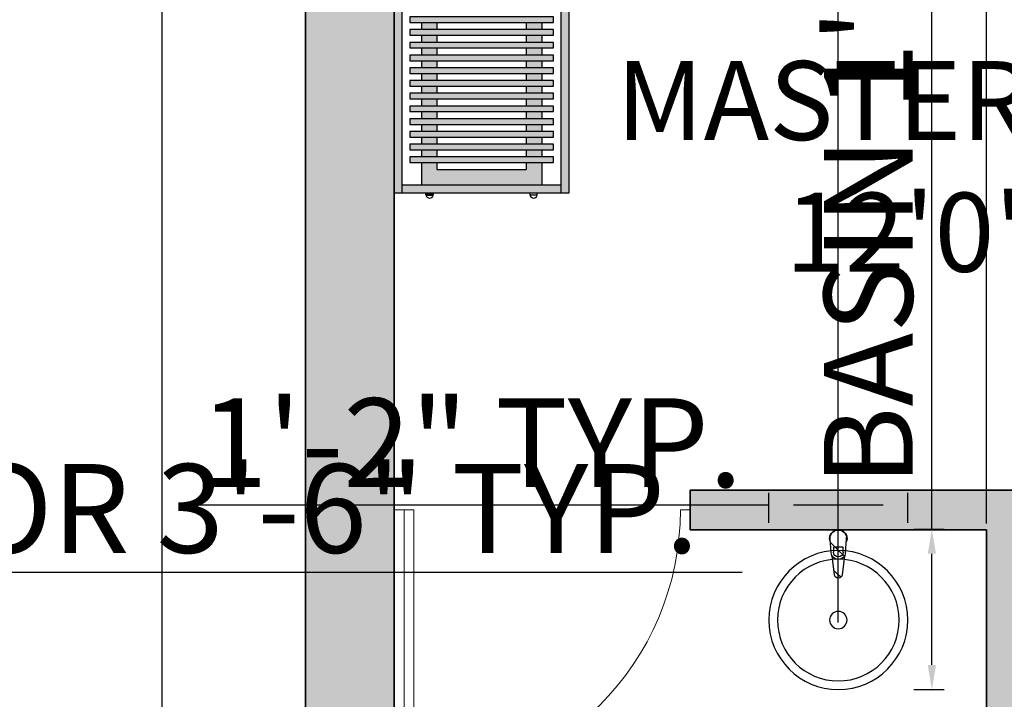
# Model space of a CAD drawing. Units: inches. Extents: x 3592 to 4861, y 1650 to 2243.
# Tile 18 of 30: x 4009 to 4109, y 2003 to 2072. Entities that reach past the tile are written whole.
import ezdxf

# ---------------------------------------------------------------- set-up
doc = ezdxf.new("R2010")
doc.units = ezdxf.units.IN
for name, color, linetype, lineweight in [('A-ANNO-DIMS', 2, 'Continuous', 13), ('A-AREA-IDEN', 7, 'Continuous', 18), ('A-DOOR', 3, 'Continuous', 20), ('A-FURN', 9, 'Continuous', 13), ('A-WALL', 7, 'Continuous', 35), ('estofado', 7, 'Continuous', 25), ('Сантехника', 9, 'Continuous', 18)]:
    doc.layers.add(name, color=color, linetype=linetype, lineweight=lineweight)
doc.layers.add('A-WALL-PATT', color=252, linetype='Continuous', lineweight=13, true_color=0x939598)
doc.layers.add('MOBIL', color=7, linetype='Continuous')
doc.layers.add('SANTEH', color=7, linetype='Continuous')
doc.styles.get("Standard").update_dxf_attribs({"font": 'arial.ttf'})
doc.dimstyles.new('ISO-25', dxfattribs={"dimtxt": 9, "dimasz": 2.5, "dimexe": 1.25, "dimexo": 0.625, "dimtad": 1, "dimlunit": 3, "dimtxsty": 'Standard', "dimcen": 2.5, "dimadec": 0, "dimazin": 0, "dimtfac": 1, "dimtmove": 0, "dimatfit": 3, "dimfxl": 1, "dimarcsym": 0})
pattern_1 = [(45, (-0.056, -259.036), (-35.355, 35.355), [])]

# ---------------------------------------------------------------- blocks, each defined once
blk = doc.blocks.new('2')
for p, q in [((3637.189, 1914.492), (3637.189, 1942.492)), ((3638.189, 1914.492), (3638.189, 1942.492)), ((3636.189, 1914.492), (3638.189, 1914.492)), ((3665.189, 1914.492), (3666.189, 1914.492))]:
    blk.add_line(p, q)
blk.add_arc((3637.189, 1914.492), 28, 0, 90)
blk = doc.blocks.new('*D6')
at = {"layer": 'A-ANNO-DIMS', "color": 0, "lineweight": -2, "transparency": 16777216}
for p, q in [((4037.745, 2165.219), (4022.592, 2165.219)), ((4023.842, 2162.719), (4023.842, 1687.719)), ((4037.745, 1685.219), (4022.592, 1685.219))]:
    blk.add_line(p, q, dxfattribs=at)
at = {"layer": 'A-ANNO-DIMS', "color": 0, "transparency": 16777216}
for points in [[(4023.426, 2162.719), (4024.259, 2162.719), (4023.842, 2165.219)], [(4023.426, 1687.719), (4024.259, 1687.719), (4023.842, 1685.219)]]:
    blk.add_solid(points, dxfattribs=at)
at = {"layer": 'Defpoints', "color": 0, "transparency": 16777216}
for p in [(4038.37, 2165.219), (4023.842, 1685.219), (4038.37, 1685.219)]:
    blk.add_point(p, dxfattribs=at)
at = {"layer": 'A-ANNO-DIMS', "color": 0, "transparency": 16777216, "insert": (4018.622, 1925.219), "char_height": 9, "attachment_point": 5, "rotation": 90}
blk.add_mtext("40'", dxfattribs=at)
blk = doc.blocks.new('r13')
at = {"layer": 'SANTEH', "ltscale": 5}
h = blk.add_hatch(dxfattribs=at)
h.set_pattern_fill('100__1', color=256, scale=0.5, angle=45, style=0)
h.set_pattern_definition(pattern_1)
h.paths.add_polyline_path([(-0.1, -138.2, -0.378173), (-11.2, -128.4), (-17.8, -75.5, -0.12102), (-21.1, -66), (-23.4, -32.9, -0.524536), (-0.1, 1)], flags=0)
h = blk.add_hatch(dxfattribs=at)
h.set_pattern_fill('100__1', color=256, scale=0.5, angle=45, style=0)
h.set_pattern_definition(pattern_1)
h.paths.add_polyline_path([(-0.1, -138.2, 0.378173), (11, -128.4), (17.7, -75.5, 0.12102), (20.9, -66), (23.3, -32.9, 0.524536), (-0.1, 1)], flags=0)
for p, q in [((-24, -25.7), (-23.9, -20.6)), ((-21.1, -66), (-24, -25.7)), ((20.9, -66), (23.8, -25.7)), ((23.8, -25.7), (23.8, -20.7)), ((-13.7, -48.9), (13.5, -48.9)), ((-13.7, -63.8), (-13.7, -48.9)), ((-13.7, -49.6), (13.5, -49.6)), ((13.5, -48.9), (13.5, -63.8)), ((-17.8, -75.5), (-11.2, -128.4)), ((11, -128.4), (17.7, -75.5))]:
    blk.add_line(p, q, dxfattribs=at)
for radius in [200, 175, 25]:
    blk.add_circle((-0.1, -259), radius, dxfattribs=at)
for centre, radius, start, end in [((-0.1, -24), 25, 339.2856, 200.7144), ((-0.1, -24), 24, 7.8374, 171.8967), ((-0.1, -63.4), 21.1, 185.1696, 354.8304), ((-0.1, -64.1), 21.1, 185.1696, 354.8304), ((-0.1, -63.8), 13.6, 180, 0), ((-0.1, -127), 11.2, 187.1389, 352.8611)]:
    blk.add_arc(centre, radius, start, end, dxfattribs=at)
blk = doc.blocks.new('Aparador Aido WV')
at = {"layer": 'MOBIL'}
h = blk.add_hatch(color=256, dxfattribs=at)
h.set_gradient(color1=(226, 228, 228), one_color=1, tint=1, name='CYLINDER')
h.paths.add_polyline_path([(0.9, -0.02), (0.9, 0), (-0.9, 0), (-0.9, -0.02)])
h = blk.add_hatch(color=256, dxfattribs=at)
h.set_gradient(color1=(226, 228, 228), one_color=1, tint=1)
h.paths.add_polyline_path([(0.9, -0.02), (0.88, -0.02), (0.88, -0.43), (0.9, -0.43)])
h = blk.add_hatch(color=256, dxfattribs=at)
h.set_gradient(color1=(106, 79, 62), color2=(55, 41, 32), one_color=1, tint=0.17)
h.paths.add_polyline_path([(0.4479, -0.0402), (0.4479, -0.4098), (0.4622, -0.4098), (0.4622, -0.0402)])
h = blk.add_hatch(color=256, dxfattribs=at)
h.set_gradient(color1=(106, 79, 62), color2=(55, 41, 32), one_color=1, tint=0.17)
h.paths.add_polyline_path([(0.4806, -0.0402), (0.4806, -0.4098), (0.495, -0.4098), (0.495, -0.0402)])
h = blk.add_hatch(color=256, dxfattribs=at)
h.set_gradient(color1=(106, 79, 62), color2=(55, 41, 32), one_color=1, tint=0.17)
h.paths.add_polyline_path([(0.5134, -0.0402), (0.5134, -0.4098), (0.5277, -0.4098), (0.5277, -0.0402)])
h = blk.add_hatch(color=256, dxfattribs=at)
h.set_gradient(color1=(106, 79, 62), color2=(55, 41, 32), one_color=1, tint=0.17)
h.paths.add_polyline_path([(0.5461, -0.0402), (0.5461, -0.4098), (0.5605, -0.4098), (0.5605, -0.0402)])
h = blk.add_hatch(color=256, dxfattribs=at)
h.set_gradient(color1=(106, 79, 62), color2=(55, 41, 32), one_color=1, tint=0.17)
h.paths.add_polyline_path([(0.5789, -0.0402), (0.5789, -0.4098), (0.5932, -0.4098), (0.5932, -0.0402)])
h = blk.add_hatch(color=256, dxfattribs=at)
h.set_gradient(color1=(106, 79, 62), color2=(55, 41, 32), one_color=1, tint=0.17)
h.paths.add_polyline_path([(0.6116, -0.0402), (0.6116, -0.4098), (0.626, -0.4098), (0.626, -0.0402)])
h = blk.add_hatch(color=256, dxfattribs=at)
h.set_gradient(color1=(106, 79, 62), color2=(55, 41, 32), one_color=1, tint=0.17)
h.paths.add_polyline_path([(0.6444, -0.0402), (0.6444, -0.4098), (0.6587, -0.4098), (0.6587, -0.0402)])
h = blk.add_hatch(color=256, dxfattribs=at)
h.set_gradient(color1=(106, 79, 62), color2=(55, 41, 32), one_color=1, tint=0.17)
h.paths.add_polyline_path([(0.6771, -0.0402), (0.6771, -0.4098), (0.6915, -0.4098), (0.6915, -0.0402)])
h = blk.add_hatch(color=256, dxfattribs=at)
h.set_gradient(color1=(106, 79, 62), color2=(55, 41, 32), one_color=1, tint=0.17)
h.paths.add_polyline_path([(0.7099, -0.0402), (0.7099, -0.4098), (0.7242, -0.4098), (0.7242, -0.0402)])
h = blk.add_hatch(color=256, dxfattribs=at)
h.set_gradient(color1=(106, 79, 62), color2=(55, 41, 32), one_color=1, tint=0.17)
h.paths.add_polyline_path([(0.7426, -0.0402), (0.7426, -0.4098), (0.757, -0.4098), (0.757, -0.0402)])
h = blk.add_hatch(color=256, dxfattribs=at)
h.set_gradient(color1=(106, 79, 62), color2=(55, 41, 32), one_color=1, tint=0.17)
h.paths.add_polyline_path([(0.7754, -0.0402), (0.7754, -0.4098), (0.7897, -0.4098), (0.7897, -0.0402)])
h = blk.add_hatch(color=256, dxfattribs=at)
h.set_gradient(color1=(106, 79, 62), color2=(55, 41, 32), one_color=1, tint=0.17)
h.paths.add_polyline_path([(0.8081, -0.0402), (0.8081, -0.4098), (0.8225, -0.4098), (0.8225, -0.0402)])
h = blk.add_hatch(color=256, dxfattribs=at)
h.set_gradient(color1=(106, 79, 62), color2=(157, 117, 92), one_color=1, tint=0.49)
h.paths.add_polyline_path([(0.4806, -0.07), (0.4622, -0.07), (0.4622, -0.11), (0.4806, -0.11)])
h = blk.add_hatch(color=256, dxfattribs=at)
h.set_gradient(color1=(106, 79, 62), color2=(157, 117, 92), one_color=1, tint=0.49)
h.paths.add_polyline_path([(0.5134, -0.07), (0.495, -0.07), (0.495, -0.11), (0.5134, -0.11)])
h = blk.add_hatch(color=256, dxfattribs=at)
h.set_gradient(color1=(106, 79, 62), color2=(157, 117, 92), one_color=1, tint=0.49)
h.paths.add_polyline_path([(0.5277, -0.11), (0.5461, -0.11), (0.5461, -0.07), (0.5277, -0.07)])
h = blk.add_hatch(color=256, dxfattribs=at)
h.set_gradient(color1=(106, 79, 62), color2=(157, 117, 92), one_color=1, tint=0.49)
h.paths.add_polyline_path([(0.5789, -0.07), (0.5605, -0.07), (0.5605, -0.11), (0.5789, -0.11)])
h = blk.add_hatch(color=256, dxfattribs=at)
h.set_gradient(color1=(106, 79, 62), color2=(157, 117, 92), one_color=1, tint=0.49)
h.paths.add_polyline_path([(0.6116, -0.07), (0.5932, -0.07), (0.5932, -0.11), (0.6116, -0.11)])
h = blk.add_hatch(color=256, dxfattribs=at)
h.set_gradient(color1=(106, 79, 62), color2=(157, 117, 92), one_color=1, tint=0.49)
h.paths.add_polyline_path([(0.6444, -0.07), (0.626, -0.07), (0.626, -0.11), (0.6444, -0.11)])
h = blk.add_hatch(color=256, dxfattribs=at)
h.set_gradient(color1=(106, 79, 62), color2=(157, 117, 92), one_color=1, tint=0.49)
h.paths.add_polyline_path([(0.6771, -0.07), (0.6587, -0.07), (0.6587, -0.11), (0.6771, -0.11)])
h = blk.add_hatch(color=256, dxfattribs=at)
h.set_gradient(color1=(106, 79, 62), color2=(157, 117, 92), one_color=1, tint=0.49)
h.paths.add_polyline_path([(0.7099, -0.07), (0.6915, -0.07), (0.6915, -0.11), (0.7099, -0.11)])
h = blk.add_hatch(color=256, dxfattribs=at)
h.set_gradient(color1=(106, 79, 62), color2=(157, 117, 92), one_color=1, tint=0.49)
h.paths.add_polyline_path([(0.7426, -0.07), (0.7242, -0.07), (0.7242, -0.11), (0.7426, -0.11)])
h = blk.add_hatch(color=256, dxfattribs=at)
h.set_gradient(color1=(106, 79, 62), color2=(157, 117, 92), one_color=1, tint=0.49)
h.paths.add_polyline_path([(0.7754, -0.07), (0.757, -0.07), (0.757, -0.11), (0.7754, -0.11)])
h = blk.add_hatch(color=256, dxfattribs=at)
h.set_gradient(color1=(106, 79, 62), color2=(157, 117, 92), one_color=1, tint=0.49)
h.paths.add_polyline_path([(0.8081, -0.07), (0.7897, -0.07), (0.7897, -0.11), (0.8081, -0.11)])
h = blk.add_hatch(color=256, dxfattribs=at)
h.set_gradient(color1=(106, 79, 62), color2=(157, 117, 92), one_color=1, tint=0.49)
h.paths.add_polyline_path([(0.88, -0.07), (0.8225, -0.07), (0.8225, -0.11), (0.84, -0.11), (0.84, -0.34), (0.8225, -0.34), (0.8225, -0.38), (0.88, -0.38)])
h = blk.add_hatch(color=256, dxfattribs=at)
h.set_gradient(color1=(106, 79, 62), color2=(157, 117, 92), one_color=1, tint=0.49)
h.paths.add_polyline_path([(0.4806, -0.34), (0.4622, -0.34), (0.4622, -0.38), (0.4806, -0.38)])
h = blk.add_hatch(color=256, dxfattribs=at)
h.set_gradient(color1=(106, 79, 62), color2=(157, 117, 92), one_color=1, tint=0.49)
h.paths.add_polyline_path([(0.5134, -0.34), (0.495, -0.34), (0.495, -0.38), (0.5134, -0.38)])
h = blk.add_hatch(color=256, dxfattribs=at)
h.set_gradient(color1=(106, 79, 62), color2=(157, 117, 92), one_color=1, tint=0.49)
h.paths.add_polyline_path([(0.5461, -0.34), (0.5277, -0.34), (0.5277, -0.38), (0.5461, -0.38)])
h = blk.add_hatch(color=256, dxfattribs=at)
h.set_gradient(color1=(106, 79, 62), color2=(157, 117, 92), one_color=1, tint=0.49)
h.paths.add_polyline_path([(0.5789, -0.34), (0.5605, -0.34), (0.5605, -0.38), (0.5789, -0.38)])
h = blk.add_hatch(color=256, dxfattribs=at)
h.set_gradient(color1=(106, 79, 62), color2=(157, 117, 92), one_color=1, tint=0.49)
h.paths.add_polyline_path([(0.6116, -0.34), (0.5932, -0.34), (0.5932, -0.38), (0.6116, -0.38)])
h = blk.add_hatch(color=256, dxfattribs=at)
h.set_gradient(color1=(106, 79, 62), color2=(157, 117, 92), one_color=1, tint=0.49)
h.paths.add_polyline_path([(0.6444, -0.34), (0.626, -0.34), (0.626, -0.38), (0.6444, -0.38)])
h = blk.add_hatch(color=256, dxfattribs=at)
h.set_gradient(color1=(106, 79, 62), color2=(157, 117, 92), one_color=1, tint=0.49)
h.paths.add_polyline_path([(0.6771, -0.34), (0.6587, -0.34), (0.6587, -0.38), (0.6771, -0.38)])
h = blk.add_hatch(color=256, dxfattribs=at)
h.set_gradient(color1=(106, 79, 62), color2=(157, 117, 92), one_color=1, tint=0.49)
h.paths.add_polyline_path([(0.7099, -0.34), (0.6915, -0.34), (0.6915, -0.38), (0.7099, -0.38)])
h = blk.add_hatch(color=256, dxfattribs=at)
h.set_gradient(color1=(106, 79, 62), color2=(157, 117, 92), one_color=1, tint=0.49)
h.paths.add_polyline_path([(0.7426, -0.34), (0.7242, -0.34), (0.7242, -0.38), (0.7426, -0.38)])
h = blk.add_hatch(color=256, dxfattribs=at)
h.set_gradient(color1=(106, 79, 62), color2=(157, 117, 92), one_color=1, tint=0.49)
h.paths.add_polyline_path([(0.7754, -0.34), (0.757, -0.34), (0.757, -0.38), (0.7754, -0.38)])
h = blk.add_hatch(color=256, dxfattribs=at)
h.set_gradient(color1=(106, 79, 62), color2=(157, 117, 92), one_color=1, tint=0.49)
h.paths.add_polyline_path([(0.8081, -0.34), (0.7897, -0.34), (0.7897, -0.38), (0.8081, -0.38)])
h = blk.add_hatch(color=256, dxfattribs=at)
h.set_gradient(color1=(226, 228, 228), one_color=1, tint=1, name='CYLINDER')
h.paths.add_polyline_path([(0.9, -0.45), (0.9, -0.43), (-0.9, -0.43), (-0.9, -0.45)])
at = {"layer": 'estofado', "ltscale": 0.5}
for p, q in [((0.4622, -0.07), (0.4806, -0.07)), ((0.495, -0.07), (0.5134, -0.07)), ((0.5277, -0.07), (0.5461, -0.07)), ((0.5605, -0.07), (0.5789, -0.07)), ((0.5932, -0.07), (0.6116, -0.07)), ((0.626, -0.07), (0.6444, -0.07)), ((0.6587, -0.07), (0.6771, -0.07)), ((0.6915, -0.07), (0.7099, -0.07)), ((0.7242, -0.07), (0.7426, -0.07)), ((0.757, -0.07), (0.7754, -0.07)), ((0.7897, -0.07), (0.8081, -0.07)), ((0.8225, -0.07), (0.88, -0.07)), ((0.9067, -0.0817), (0.9067, -0.1006)), ((0.4622, -0.11), (0.4806, -0.11)), ((0.495, -0.11), (0.5134, -0.11)), ((0.5277, -0.11), (0.5461, -0.11)), ((0.5605, -0.11), (0.5789, -0.11)), ((0.5932, -0.11), (0.6116, -0.11)), ((0.626, -0.11), (0.6444, -0.11)), ((0.6587, -0.11), (0.6771, -0.11)), ((0.6915, -0.11), (0.7099, -0.11)), ((0.7242, -0.11), (0.7426, -0.11)), ((0.757, -0.11), (0.7754, -0.11)), ((0.7897, -0.11), (0.8081, -0.11)), ((0.8225, -0.11), (0.84, -0.11)), ((0.84, -0.34), (0.84, -0.11)), ((0.4622, -0.34), (0.4806, -0.34)), ((0.495, -0.34), (0.5134, -0.34)), ((0.5277, -0.34), (0.5461, -0.34)), ((0.5605, -0.34), (0.5789, -0.34)), ((0.5932, -0.34), (0.6116, -0.34)), ((0.626, -0.34), (0.6444, -0.34)), ((0.6587, -0.34), (0.6771, -0.34)), ((0.6915, -0.34), (0.7099, -0.34)), ((0.7242, -0.34), (0.7426, -0.34)), ((0.757, -0.34), (0.7754, -0.34)), ((0.7897, -0.34), (0.8081, -0.34)), ((0.8225, -0.34), (0.84, -0.34)), ((0.9067, -0.3683), (0.9067, -0.3494)), ((0.4622, -0.38), (0.4806, -0.38)), ((0.495, -0.38), (0.5134, -0.38)), ((0.5277, -0.38), (0.5461, -0.38)), ((0.5605, -0.38), (0.5789, -0.38)), ((0.5932, -0.38), (0.6116, -0.38)), ((0.626, -0.38), (0.6444, -0.38)), ((0.6587, -0.38), (0.6771, -0.38)), ((0.6915, -0.38), (0.7099, -0.38)), ((0.7242, -0.38), (0.7426, -0.38)), ((0.757, -0.38), (0.7754, -0.38)), ((0.7897, -0.38), (0.8081, -0.38)), ((0.8225, -0.38), (0.88, -0.38))]:
    blk.add_line(p, q, dxfattribs=at)
for points in [[(0.4479, -0.0402), (0.4479, -0.4098), (0.4622, -0.4098), (0.4622, -0.0402)], [(0.4806, -0.0402), (0.4806, -0.4098), (0.495, -0.4098), (0.495, -0.0402)], [(0.5134, -0.0402), (0.5134, -0.4098), (0.5277, -0.4098), (0.5277, -0.0402)], [(0.5461, -0.0402), (0.5461, -0.4098), (0.5605, -0.4098), (0.5605, -0.0402)], [(0.5789, -0.0402), (0.5789, -0.4098), (0.5932, -0.4098), (0.5932, -0.0402)], [(0.6116, -0.0402), (0.6116, -0.4098), (0.626, -0.4098), (0.626, -0.0402)], [(0.6444, -0.0402), (0.6444, -0.4098), (0.6587, -0.4098), (0.6587, -0.0402)], [(0.6771, -0.0402), (0.6771, -0.4098), (0.6915, -0.4098), (0.6915, -0.0402)], [(0.7099, -0.0402), (0.7099, -0.4098), (0.7242, -0.4098), (0.7242, -0.0402)], [(0.7426, -0.0402), (0.7426, -0.4098), (0.757, -0.4098), (0.757, -0.0402)], [(0.7754, -0.0402), (0.7754, -0.4098), (0.7897, -0.4098), (0.7897, -0.0402)], [(0.8081, -0.0402), (0.8081, -0.4098), (0.8225, -0.4098), (0.8225, -0.0402)], [(0.9054, -0.0817), (0.9009, -0.0817), (0.9009, -0.1006), (0.9054, -0.1006)], [(0.9054, -0.3683), (0.9009, -0.3683), (0.9009, -0.3494), (0.9054, -0.3494)]]:
    blk.add_lwpolyline(points, close=True, dxfattribs=at)
for centre in [(0.904, -0.0911), (0.904, -0.3589)]:
    blk.add_arc(centre, 0.0098, 285.9849, 74.0151, dxfattribs=at)
at = {"layer": 'MOBIL'}
for p, q in [((0.9, -0.02), (-0.9, -0.02)), ((0.88, -0.43), (0.88, -0.02)), ((-0.9, -0.43), (0.9, -0.43))]:
    blk.add_line(p, q, dxfattribs=at)
blk.add_lwpolyline([(-0.9, -0.45), (0.9, -0.45), (0.9, 0), (-0.9, 0)], close=True, dxfattribs=at)
blk = doc.blocks.new('*D142')
at = {"layer": 'A-ANNO-DIMS', "color": 0, "lineweight": -2, "transparency": 16777216}
for p, q in [((3886.061, 2021.594), (3886.061, 2014.669)), ((3928.061, 2021.594), (3928.061, 2014.669)), ((3888.561, 2015.919), (3925.561, 2015.919)), ((3928.061, 2015.919), (4082.632, 2015.919))]:
    blk.add_line(p, q, dxfattribs=at)
at = {"layer": 'A-ANNO-DIMS', "color": 0, "transparency": 16777216}
for points in [[(3888.561, 2016.336), (3888.561, 2015.502), (3886.061, 2015.919)], [(3925.561, 2016.336), (3925.561, 2015.502), (3928.061, 2015.919)]]:
    blk.add_solid(points, dxfattribs=at)
at = {"layer": 'Defpoints', "color": 0, "transparency": 16777216}
for p in [(3886.061, 2022.219), (3928.061, 2022.219), (3928.061, 2015.919)]:
    blk.add_point(p, dxfattribs=at)
at = {"layer": 'A-ANNO-DIMS', "color": 0, "transparency": 16777216, "insert": (4006.597, 2021.204), "char_height": 9, "attachment_point": 5}
blk.add_mtext('DOUBLE DOOR 3\'-6" TYP.', dxfattribs=at)
blk = doc.blocks.new('*D150')
at = {"layer": 'A-ANNO-DIMS', "color": 0, "lineweight": -2, "transparency": 16777216}
for p, q in [((4101.85, 2020.278), (4101.85, 2140.684)), ((4100.037, 2020.278), (4103.1, 2020.278)), ((4101.85, 2006.522), (4101.85, 2017.778)), ((4100.037, 2004.022), (4103.1, 2004.022))]:
    blk.add_line(p, q, dxfattribs=at)
at = {"layer": 'A-ANNO-DIMS', "color": 0, "transparency": 16777216}
for points in [[(4101.433, 2017.778), (4102.267, 2017.778), (4101.85, 2020.278)], [(4101.433, 2006.522), (4102.267, 2006.522), (4101.85, 2004.022)]]:
    blk.add_solid(points, dxfattribs=at)
at = {"layer": 'Defpoints', "color": 0, "transparency": 16777216}
for p in [(4099.412, 2020.278), (4101.85, 2020.278), (4099.412, 2004.022)]:
    blk.add_point(p, dxfattribs=at)
at = {"layer": 'A-ANNO-DIMS', "color": 0, "transparency": 16777216, "insert": (4096.571, 2081.731), "char_height": 9, "attachment_point": 5, "rotation": 90}
blk.add_mtext('BASIN 1\'-4 1/2" TYP.', dxfattribs=at)
blk = doc.blocks.new('*D151')
at = {"layer": 'A-ANNO-DIMS', "color": 0, "lineweight": -2, "transparency": 16777216}
for p, q in [((4085.328, 2020.903), (4085.328, 2023.966)), ((4099.412, 2020.903), (4099.412, 2023.966)), ((4085.328, 2022.716), (4027.565, 2022.716)), ((4096.912, 2022.716), (4087.828, 2022.716))]:
    blk.add_line(p, q, dxfattribs=at)
at = {"layer": 'A-ANNO-DIMS', "color": 0, "transparency": 16777216}
for points in [[(4087.828, 2023.133), (4087.828, 2022.299), (4085.328, 2022.716)], [(4096.912, 2023.133), (4096.912, 2022.299), (4099.412, 2022.716)]]:
    blk.add_solid(points, dxfattribs=at)
at = {"layer": 'Defpoints', "color": 0, "transparency": 16777216}
for p in [(4085.328, 2022.716), (4085.328, 2020.278), (4099.412, 2020.278)]:
    blk.add_point(p, dxfattribs=at)
at = {"layer": 'A-ANNO-DIMS', "color": 0, "transparency": 16777216, "insert": (4055.197, 2027.863), "char_height": 9, "attachment_point": 5}
blk.add_mtext('1\'-2" TYP.', dxfattribs=at)
blk = doc.blocks.new('*D179')
at = {"layer": 'A-ANNO-DIMS', "color": 0, "lineweight": -2, "transparency": 16777216}
for p, q in [((4092.37, 2010.809), (4092.37, 2193.519)), ((4107.37, 2020.844), (4107.37, 2193.519)), ((4094.87, 2192.269), (4104.87, 2192.269)), ((4107.37, 2192.269), (4134.197, 2192.269))]:
    blk.add_line(p, q, dxfattribs=at)
at = {"layer": 'A-ANNO-DIMS', "color": 0, "transparency": 16777216}
for points in [[(4094.87, 2192.686), (4094.87, 2191.852), (4092.37, 2192.269)], [(4104.87, 2192.686), (4104.87, 2191.852), (4107.37, 2192.269)]]:
    blk.add_solid(points, dxfattribs=at)
at = {"layer": 'Defpoints', "color": 0, "transparency": 16777216}
for p in [(4107.37, 2192.269), (4107.37, 2020.219), (4092.37, 2010.184)]:
    blk.add_point(p, dxfattribs=at)
at = {"layer": 'A-ANNO-DIMS', "color": 0, "transparency": 16777216, "insert": (4122.033, 2197.492), "char_height": 9, "attachment_point": 5}
blk.add_mtext('1\'-3"', dxfattribs=at)

msp = doc.modelspace()

# ---------------------------------------------------------------- hatches: boundary and pattern name
at = {"layer": 'A-WALL-PATT'}
h = msp.add_hatch(color=256, dxfattribs=at)
h.dxf.hatch_style = 1
h.paths.add_polyline_path([(4398.37, 2165.219), (4038.37, 2165.219), (4038.37, 1993.219), (4047.37, 1993.219), (4047.37, 2156.219), (4191.37, 2156.219), (4191.37, 2150.219), (4195.37, 2150.219), (4195.37, 2156.219), (4256.37, 2156.219), (4256.37, 2150.219), (4265.37, 2150.219), (4265.37, 2156.219), (4389.37, 2156.219), (4389.37, 2114.219), (4398.37, 2114.219)])
h.paths.add_polyline_path([(4265.37, 2102.219), (4256.37, 2102.219), (4256.37, 2096.219), (4195.37, 2096.219), (4195.37, 2102.219), (4191.37, 2102.219), (4191.37, 2020.219), (4195.37, 2020.219), (4195.37, 2087.219), (4256.37, 2087.219), (4256.37, 2020.219), (4306.37, 2020.219), (4306.37, 2024.219), (4265.37, 2024.219)], flags=17)
h.paths.add_polyline_path([(4398.37, 2066.219), (4389.37, 2066.219), (4389.37, 2024.219), (4348.37, 2024.219), (4348.37, 2020.219), (4389.37, 2020.219), (4389.37, 1989.719), (4398.37, 1989.719)])
h.paths.add_polyline_path([(4398.37, 1941.719), (4389.37, 1941.719), (4389.37, 1911.219), (4301.37, 1911.219), (4301.37, 1907.219), (4389.37, 1907.219), (4389.37, 1865.219), (4398.37, 1865.219)])
h.paths.add_polyline_path([(4398.37, 1817.219), (4389.37, 1817.219), (4389.37, 1775.219), (4265.37, 1775.219), (4265.37, 1911.219), (4256.37, 1911.219), (4256.37, 1817.219), (4220.87, 1817.219), (4220.87, 1808.219), (4256.37, 1808.219), (4256.37, 1766.219), (4389.37, 1766.219), (4389.37, 1694.219), (4256.37, 1694.219), (4256.37, 1685.219), (4398.37, 1685.219)])
h.paths.add_polyline_path([(4178.87, 1817.219), (4077.37, 1817.219), (4077.37, 1808.219), (4178.87, 1808.219)])
h.paths.add_polyline_path([(4111.37, 2020.219), (4155.37, 2020.219), (4155.37, 2024.219), (4077.37, 2024.219), (4077.37, 2020.219), (4107.37, 2020.219), (4107.37, 1942.219), (4047.37, 1942.219), (4047.37, 1969.219), (4038.37, 1969.219), (4038.37, 1911.219), (4047.37, 1911.219), (4047.37, 1938.219), (4107.37, 1938.219), (4107.37, 1860.219), (4077.37, 1860.219), (4077.37, 1856.219), (4111.37, 1856.219)])
h.paths.add_polyline_path([(4047.37, 1887.219), (4038.37, 1887.219), (4038.37, 1685.219), (4152.37, 1685.219), (4152.37, 1715.219), (4143.37, 1715.219), (4143.37, 1694.219), (4047.37, 1694.219)])
h.paths.add_polyline_path([(4152.37, 1772.219), (4143.37, 1772.219), (4143.37, 1751.219), (4152.37, 1751.219)], flags=17)

# ---------------------------------------------------------------- linework, layer by layer
at = {"layer": 'A-WALL'}
for p, q in [((4038.37, 1685.219), (4038.37, 2165.219)), ((4047.37, 1942.219), (4047.37, 2156.219)), ((4077.37, 2024.219), (4155.37, 2024.219)), ((4077.37, 2020.219), (4077.37, 2024.219)), ((4077.37, 2020.219), (4107.37, 2020.219)), ((4107.37, 1942.219), (4107.37, 2020.219))]:
    msp.add_line(p, q, dxfattribs=at)

# ---------------------------------------------------------------- block references
at = {"layer": 'A-DOOR', "xscale": -1, "rotation": 180}
msp.add_blockref('2', (411.181, 3936.711), dxfattribs=at)
at = {"layer": 'A-FURN', "xscale": 39.3701, "yscale": 39.3701, "zscale": 39.3701, "rotation": 270}
msp.add_blockref('Aparador Aido WV', (4065.086, 2089.784), dxfattribs=at)
at = {"layer": 'Сантехника', "xscale": -0.0352097458701181, "yscale": 0.0352097458701181, "zscale": 0.0352097458701181}
msp.add_blockref('r13', (4092.368, 2020.185), dxfattribs=at)

# ---------------------------------------------------------------- texts
at = {"layer": 'A-AREA-IDEN', "insert": (4069.864, 2067.679), "char_height": 8, "attachment_point": 1}
msp.add_mtext_dynamic_manual_height_columns('MASTER BEDROOM\\P       12\'0"X11\'0"', width=121.44943, gutter_width=12.5, heights=[0], dxfattribs=at)

# ---------------------------------------------------------------- dimensions: what is measured, and where the dimension line sits
at = {"layer": 'A-ANNO-DIMS'}
dim = msp.add_linear_dim(base=(4107.37, 2192.269), p1=(4092.37, 2010.184), p2=(4107.37, 2020.219), dimstyle='ISO-25', override={"dimdec": 1, "dimlfac": 1, "dimrnd": 0, "dimzin": 1, "dimdsep": 46, "dimlunit": 4, "dimfrac": 2}, dxfattribs=at)
dim.commit()
dim.dimension.update_dxf_attribs({"geometry": '*D179', "text_midpoint": (4122.033, 2197.492)})
dim = msp.add_linear_dim(base=(4023.842, 1685.219), p1=(4038.37, 2165.219), p2=(4038.37, 1685.219), angle=90, dimstyle='ISO-25', override={"dimclrd": 0, "dimclre": 0, "dimclrt": 0}, dxfattribs=at)
dim.commit()
dim.dimension.update_dxf_attribs({"geometry": '*D6', "text_midpoint": (4018.622, 1925.219)})
for base, p1, p2, angle, text, picture, middle in [((4101.85, 2020.278), (4099.412, 2004.022), (4099.412, 2020.278), 90, 'BASIN <> TYP.', '*D150', (4096.571, 2081.731)), ((4085.328, 2022.716), (4099.412, 2020.278), (4085.328, 2020.278), 180, '<> TYP.', '*D151', (4055.197, 2027.863))]:
    dim = msp.add_linear_dim(base=base, p1=p1, p2=p2, angle=angle, text=text, dimstyle='ISO-25', override={"dimdec": 1, "dimlfac": 1, "dimrnd": 0, "dimzin": 1, "dimdsep": 46, "dimlunit": 4, "dimfrac": 2}, dxfattribs=at)
    dim.commit()
    dim.dimension.update_dxf_attribs({"geometry": picture, "text_midpoint": middle})
dim = msp.add_linear_dim(base=(3928.061, 2015.919), p1=(3886.061, 2022.219), p2=(3928.061, 2022.219), text='DOUBLE DOOR <> TYP.', dimstyle='ISO-25', override={"dimdec": 1, "dimlfac": 1, "dimrnd": 0, "dimzin": 1, "dimdsep": 46, "dimlunit": 4, "dimfrac": 2}, dxfattribs=at)
dim.commit()
dim.dimension.update_dxf_attribs({"geometry": '*D142', "text_midpoint": (4006.597, 2021.204)})

doc.saveas('drawing.dxf')
